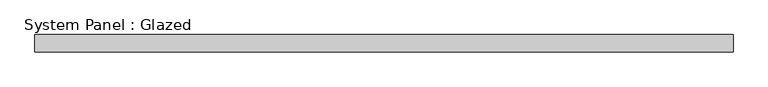
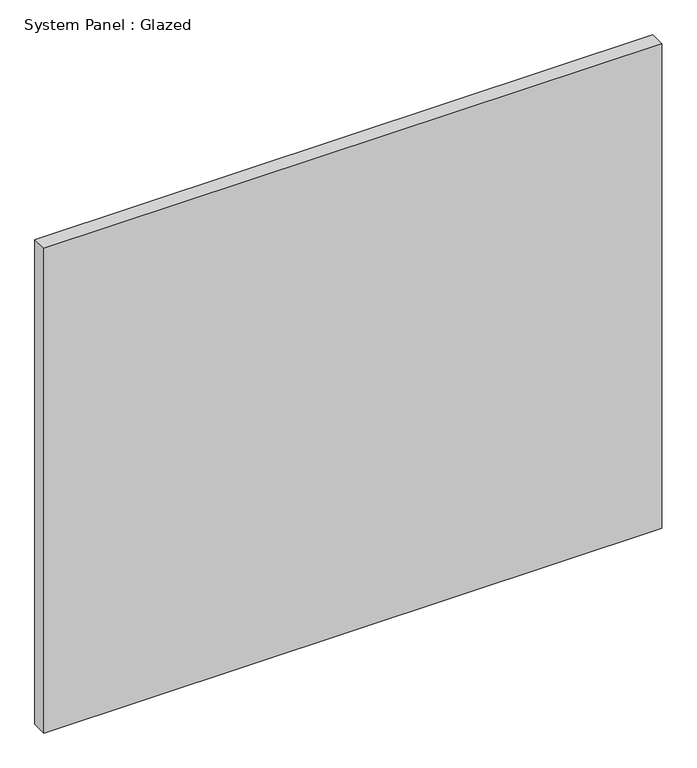
"""IFC4 building model written with IfcOpenShell, lengths in millimetres: plate geometry, System Panel : Glazed."""

from ifc_helpers import new_model, si_unit, origin, origin_with_axes, place, context, project, spatial, polyline, outline, extrude, source, transform, mapped, element, save


def system_panel_glazed_a6fb9a4f(model_context):
    return source(origin(), model_context, "Body", "SweptSolid", [
        extrude(outline(polyline([(514.35, 19.05), (-514.35, 19.05), (-514.35, 44.45), (514.35, 44.45), (514.35, 19.05)])), origin_with_axes(), (0.0, 0.0, 1.0), 853.0145651),
    ])


if __name__ == "__main__":
    model = new_model("IFC4")
    model_context = context("Model", 3, world=origin())
    ifc_project = project(units=[si_unit("LENGTHUNIT", "METRE", prefix="MILLI")], contexts=[model_context])
    site = spatial("IfcSite", under=ifc_project)
    building = spatial("IfcBuilding", under=site)
    placement = place(None, origin())
    system_panel_glazed_shape = system_panel_glazed_a6fb9a4f(model_context)
    element("IfcPlate", 1, ObjectType="System Panel : Glazed", at=placement, inside=building, context=model_context, shape_type="MappedRepresentation", body=[
        mapped(system_panel_glazed_shape, transform((0.0, 0.0, 0.0), x_axis=(1.0, 0.0, 0.0), y_axis=(0.0, 1.0, 0.0), z_axis=(0.0, 0.0, 1.0))),
    ])
    save(model, "model.ifc")

# Revit data of these elements
# Type "System Panel : Glazed"
#   Construction Type Id = "GSP4R"
#   Analytic Construction = "1/8 in Pilkington single glazing"
#   Visual Light Transmittance = 0.9
#   Solar Heat Gain Coefficient = 0.86
#   Heat Transfer Coefficient (U) = 1.18115 BTU/(h·ft²·°F)
#   Define Thermal Properties by = 1
# Element 1 (IfcPlate, "System Panel : Glazed")
#   Materials on its faces: "Glass"
# Materials
#   "Glass": class "Glass", colour RGB 0 128 192, transparency 0.75, Description = "Soda Lime Glass", Cost = 0
